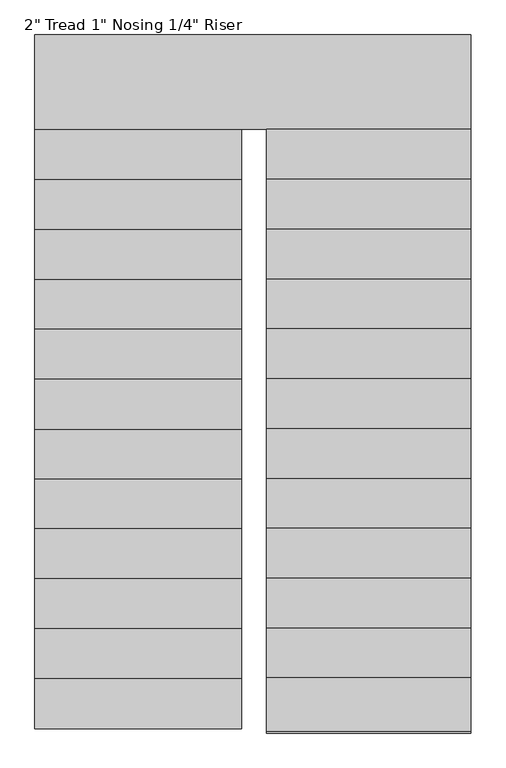
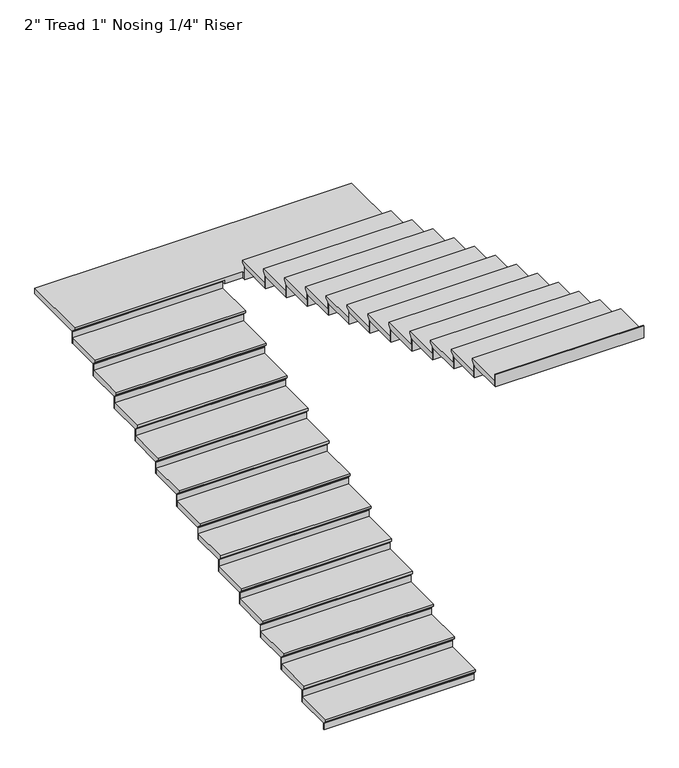
"""IFC4 building model written with IfcOpenShell, lengths in millimetres: stair flight geometry."""

from ifc_helpers import new_model, si_unit, origin, place, context, project, spatial, faceted_brep, source, transform, mapped, element, save


def stair_flight_f068cff5(model_context):
    return source(origin(), model_context, "Body", "Brep", [
        faceted_brep([(-2593.7381751, -9955.5916506, 21422.4576923), (-2593.7381751, -9955.5916506, 21441.5076923), (-3857.687215, -9955.5916506, 21441.5076923), (-3857.687215, -9955.5916506, 21422.4576923), (-2593.7381751, -9930.1916506, 21397.0576923), (-3857.687215, -9930.1916506, 21397.0576923), (-2593.7381751, -9619.0416506, 21441.5076923), (-3857.687215, -9619.0416506, 21441.5076923), (-3857.687215, -9930.1916506, 21390.7076923), (-3857.687215, -9619.0416506, 21390.7076923), (-2593.7381751, -9619.0416506, 21390.7076923), (-2593.7381751, -9930.1916506, 21390.7076923)], [[[0, 1, 2, 3]], [[4, 0, 3, 5]], [[2, 1, 6, 7]], [[8, 9, 10, 11]], [[2, 7, 9, 8, 5, 3]], [[8, 11, 4, 5]], [[6, 1, 0, 4, 11, 10]], [[7, 6, 10, 9]]]),
        faceted_brep([(-2593.7381751, -9930.1916506, 21390.7076923), (-2593.7381751, -9930.1916506, 21336.0), (-2593.7381751, -9923.8416506, 21336.0), (-2593.7381751, -9923.8416506, 21390.7076923), (-3857.687215, -9930.1916506, 21390.7076923), (-3857.687215, -9923.8416506, 21390.7076923), (-3857.687215, -9923.8416506, 21336.0), (-3857.687215, -9930.1916506, 21336.0)], [[[0, 1, 2, 3]], [[4, 5, 6, 7]], [[1, 0, 4, 7]], [[2, 1, 7, 6]], [[3, 2, 6, 5]], [[0, 3, 5, 4]]]),
        faceted_brep([(-2593.7381751, -9619.0416506, 21496.2153846), (-2593.7381751, -9619.0416506, 21390.7076923), (-2593.7381751, -9612.6916506, 21390.7076923), (-2593.7381751, -9612.6916506, 21496.2153846), (-3857.687215, -9619.0416506, 21496.2153846), (-3857.687215, -9612.6916506, 21496.2153846), (-3857.687215, -9612.6916506, 21390.7076923), (-3857.687215, -9619.0416506, 21390.7076923)], [[[0, 1, 2, 3]], [[4, 5, 6, 7]], [[1, 0, 4, 7]], [[2, 1, 7, 6]], [[3, 2, 6, 5]], [[0, 3, 5, 4]]]),
        faceted_brep([(-3857.687215, -9644.4416506, 21547.0153846), (-2593.7381751, -9644.4416506, 21547.0153846), (-2593.7381751, -9314.2416506, 21547.0153846), (-3857.687215, -9314.2416506, 21547.0153846), (-3857.687215, -9619.0416506, 21496.2153846), (-3857.687215, -9314.2416506, 21496.2153846), (-2593.7381751, -9314.2416506, 21496.2153846), (-2593.7381751, -9619.0416506, 21496.2153846), (-3857.687215, -9619.0416506, 21502.5653846), (-3857.687215, -9644.4416506, 21527.9653846), (-2593.7381751, -9619.0416506, 21502.5653846), (-2593.7381751, -9644.4416506, 21527.9653846)], [[[0, 1, 2, 3]], [[4, 5, 6, 7]], [[0, 3, 5, 4, 8, 9]], [[4, 7, 10, 8]], [[2, 1, 11, 10, 7, 6]], [[3, 2, 6, 5]], [[11, 1, 0, 9]], [[10, 11, 9, 8]]]),
        faceted_brep([(-2593.7381751, -9314.2416506, 21601.7230769), (-2593.7381751, -9314.2416506, 21496.2153846), (-2593.7381751, -9307.8916506, 21496.2153846), (-2593.7381751, -9307.8916506, 21601.7230769), (-3857.687215, -9314.2416506, 21601.7230769), (-3857.687215, -9307.8916506, 21601.7230769), (-3857.687215, -9307.8916506, 21496.2153846), (-3857.687215, -9314.2416506, 21496.2153846)], [[[0, 1, 2, 3]], [[4, 5, 6, 7]], [[1, 0, 4, 7]], [[2, 1, 7, 6]], [[3, 2, 6, 5]], [[0, 3, 5, 4]]]),
        faceted_brep([(-3857.687215, -9339.6416506, 21652.5230769), (-2593.7381751, -9339.6416506, 21652.5230769), (-2593.7381751, -9009.4416506, 21652.5230769), (-3857.687215, -9009.4416506, 21652.5230769), (-3857.687215, -9314.2416506, 21601.7230769), (-3857.687215, -9009.4416506, 21601.7230769), (-2593.7381751, -9009.4416506, 21601.7230769), (-2593.7381751, -9314.2416506, 21601.7230769), (-3857.687215, -9314.2416506, 21608.0730769), (-3857.687215, -9339.6416506, 21633.4730769), (-2593.7381751, -9314.2416506, 21608.0730769), (-2593.7381751, -9339.6416506, 21633.4730769)], [[[0, 1, 2, 3]], [[4, 5, 6, 7]], [[0, 3, 5, 4, 8, 9]], [[4, 7, 10, 8]], [[2, 1, 11, 10, 7, 6]], [[3, 2, 6, 5]], [[11, 1, 0, 9]], [[10, 11, 9, 8]]]),
        faceted_brep([(-2593.7381751, -9009.4416506, 21707.2307692), (-2593.7381751, -9009.4416506, 21601.7230769), (-2593.7381751, -9003.0916506, 21601.7230769), (-2593.7381751, -9003.0916506, 21707.2307692), (-3857.687215, -9009.4416506, 21707.2307692), (-3857.687215, -9003.0916506, 21707.2307692), (-3857.687215, -9003.0916506, 21601.7230769), (-3857.687215, -9009.4416506, 21601.7230769)], [[[0, 1, 2, 3]], [[4, 5, 6, 7]], [[1, 0, 4, 7]], [[2, 1, 7, 6]], [[3, 2, 6, 5]], [[0, 3, 5, 4]]]),
        faceted_brep([(-3857.687215, -9034.8416506, 21758.0307692), (-2593.7381751, -9034.8416506, 21758.0307692), (-2593.7381751, -8704.6416506, 21758.0307692), (-3857.687215, -8704.6416506, 21758.0307692), (-3857.687215, -9009.4416506, 21707.2307692), (-3857.687215, -8704.6416506, 21707.2307692), (-2593.7381751, -8704.6416506, 21707.2307692), (-2593.7381751, -9009.4416506, 21707.2307692), (-3857.687215, -9009.4416506, 21713.5807692), (-3857.687215, -9034.8416506, 21738.9807692), (-2593.7381751, -9009.4416506, 21713.5807692), (-2593.7381751, -9034.8416506, 21738.9807692)], [[[0, 1, 2, 3]], [[4, 5, 6, 7]], [[0, 3, 5, 4, 8, 9]], [[4, 7, 10, 8]], [[2, 1, 11, 10, 7, 6]], [[3, 2, 6, 5]], [[11, 1, 0, 9]], [[10, 11, 9, 8]]]),
        faceted_brep([(-2593.7381751, -8704.6416506, 21812.7384615), (-2593.7381751, -8704.6416506, 21707.2307692), (-2593.7381751, -8698.2916506, 21707.2307692), (-2593.7381751, -8698.2916506, 21812.7384615), (-3857.687215, -8704.6416506, 21812.7384615), (-3857.687215, -8698.2916506, 21812.7384615), (-3857.687215, -8698.2916506, 21707.2307692), (-3857.687215, -8704.6416506, 21707.2307692)], [[[0, 1, 2, 3]], [[4, 5, 6, 7]], [[1, 0, 4, 7]], [[2, 1, 7, 6]], [[3, 2, 6, 5]], [[0, 3, 5, 4]]]),
        faceted_brep([(-3857.687215, -8730.0416506, 21863.5384615), (-2593.7381751, -8730.0416506, 21863.5384615), (-2593.7381751, -8399.8416506, 21863.5384615), (-3857.687215, -8399.8416506, 21863.5384615), (-3857.687215, -8704.6416506, 21812.7384615), (-3857.687215, -8399.8416506, 21812.7384615), (-2593.7381751, -8399.8416506, 21812.7384615), (-2593.7381751, -8704.6416506, 21812.7384615), (-3857.687215, -8704.6416506, 21819.0884615), (-3857.687215, -8730.0416506, 21844.4884615), (-2593.7381751, -8704.6416506, 21819.0884615), (-2593.7381751, -8730.0416506, 21844.4884615)], [[[0, 1, 2, 3]], [[4, 5, 6, 7]], [[0, 3, 5, 4, 8, 9]], [[4, 7, 10, 8]], [[2, 1, 11, 10, 7, 6]], [[3, 2, 6, 5]], [[11, 1, 0, 9]], [[10, 11, 9, 8]]]),
        faceted_brep([(-2593.7381751, -8399.8416506, 21918.2461538), (-2593.7381751, -8399.8416506, 21812.7384615), (-2593.7381751, -8393.4916506, 21812.7384615), (-2593.7381751, -8393.4916506, 21918.2461538), (-3857.687215, -8399.8416506, 21918.2461538), (-3857.687215, -8393.4916506, 21918.2461538), (-3857.687215, -8393.4916506, 21812.7384615), (-3857.687215, -8399.8416506, 21812.7384615)], [[[0, 1, 2, 3]], [[4, 5, 6, 7]], [[1, 0, 4, 7]], [[2, 1, 7, 6]], [[3, 2, 6, 5]], [[0, 3, 5, 4]]]),
        faceted_brep([(-3857.687215, -8425.2416506, 21969.0461538), (-2593.7381751, -8425.2416506, 21969.0461538), (-2593.7381751, -8098.2166506, 21969.0461538), (-3857.687215, -8098.2166506, 21969.0461538), (-3857.687215, -8399.8416506, 21918.2461538), (-3857.687215, -8098.2166506, 21918.2461538), (-2593.7381751, -8098.2166506, 21918.2461538), (-2593.7381751, -8399.8416506, 21918.2461538), (-3857.687215, -8399.8416506, 21924.5961538), (-3857.687215, -8425.2416506, 21949.9961538), (-2593.7381751, -8399.8416506, 21924.5961538), (-2593.7381751, -8425.2416506, 21949.9961538)], [[[0, 1, 2, 3]], [[4, 5, 6, 7]], [[0, 3, 5, 4, 8, 9]], [[4, 7, 10, 8]], [[2, 1, 11, 10, 7, 6]], [[3, 2, 6, 5]], [[11, 1, 0, 9]], [[10, 11, 9, 8]]]),
        faceted_brep([(-2593.7381751, -8098.2166506, 22023.7538462), (-2593.7381751, -8098.2166506, 21918.2461538), (-2593.7381751, -8091.8666506, 21918.2461538), (-2593.7381751, -8091.8666506, 22023.7538462), (-3857.687215, -8098.2166506, 22023.7538462), (-3857.687215, -8091.8666506, 22023.7538462), (-3857.687215, -8091.8666506, 21918.2461538), (-3857.687215, -8098.2166506, 21918.2461538)], [[[0, 1, 2, 3]], [[4, 5, 6, 7]], [[1, 0, 4, 7]], [[2, 1, 7, 6]], [[3, 2, 6, 5]], [[0, 3, 5, 4]]]),
        faceted_brep([(-3857.687215, -8123.6166506, 22074.5538462), (-2593.7381751, -8123.6166506, 22074.5538462), (-2593.7381751, -7790.2416506, 22074.5538462), (-3857.687215, -7790.2416506, 22074.5538462), (-3857.687215, -8098.2166506, 22023.7538462), (-3857.687215, -7790.2416506, 22023.7538462), (-2593.7381751, -7790.2416506, 22023.7538462), (-2593.7381751, -8098.2166506, 22023.7538462), (-3857.687215, -8098.2166506, 22030.1038462), (-3857.687215, -8123.6166506, 22055.5038462), (-2593.7381751, -8098.2166506, 22030.1038462), (-2593.7381751, -8123.6166506, 22055.5038462)], [[[0, 1, 2, 3]], [[4, 5, 6, 7]], [[0, 3, 5, 4, 8, 9]], [[4, 7, 10, 8]], [[2, 1, 11, 10, 7, 6]], [[3, 2, 6, 5]], [[11, 1, 0, 9]], [[10, 11, 9, 8]]]),
        faceted_brep([(-2593.7381751, -7790.2416506, 22129.2615385), (-2593.7381751, -7790.2416506, 22023.7538462), (-2593.7381751, -7783.8916506, 22023.7538462), (-2593.7381751, -7783.8916506, 22129.2615385), (-3857.687215, -7790.2416506, 22129.2615385), (-3857.687215, -7783.8916506, 22129.2615385), (-3857.687215, -7783.8916506, 22023.7538462), (-3857.687215, -7790.2416506, 22023.7538462)], [[[0, 1, 2, 3]], [[4, 5, 6, 7]], [[1, 0, 4, 7]], [[2, 1, 7, 6]], [[3, 2, 6, 5]], [[0, 3, 5, 4]]]),
        faceted_brep([(-3857.687215, -7815.6416506, 22180.0615385), (-2593.7381751, -7815.6416506, 22180.0615385), (-2593.7381751, -7485.4416506, 22180.0615385), (-3857.687215, -7485.4416506, 22180.0615385), (-3857.687215, -7790.2416506, 22129.2615385), (-3857.687215, -7485.4416506, 22129.2615385), (-2593.7381751, -7485.4416506, 22129.2615385), (-2593.7381751, -7790.2416506, 22129.2615385), (-3857.687215, -7790.2416506, 22135.6115385), (-3857.687215, -7815.6416506, 22161.0115385), (-2593.7381751, -7790.2416506, 22135.6115385), (-2593.7381751, -7815.6416506, 22161.0115385)], [[[0, 1, 2, 3]], [[4, 5, 6, 7]], [[0, 3, 5, 4, 8, 9]], [[4, 7, 10, 8]], [[2, 1, 11, 10, 7, 6]], [[3, 2, 6, 5]], [[11, 1, 0, 9]], [[10, 11, 9, 8]]]),
        faceted_brep([(-2593.7381751, -7485.4416506, 22234.7692308), (-2593.7381751, -7485.4416506, 22129.2615385), (-2593.7381751, -7479.0916506, 22129.2615385), (-2593.7381751, -7479.0916506, 22234.7692308), (-3857.687215, -7485.4416506, 22234.7692308), (-3857.687215, -7479.0916506, 22234.7692308), (-3857.687215, -7479.0916506, 22129.2615385), (-3857.687215, -7485.4416506, 22129.2615385)], [[[0, 1, 2, 3]], [[4, 5, 6, 7]], [[1, 0, 4, 7]], [[2, 1, 7, 6]], [[3, 2, 6, 5]], [[0, 3, 5, 4]]]),
        faceted_brep([(-3857.687215, -7510.8416506, 22285.5692308), (-2593.7381751, -7510.8416506, 22285.5692308), (-2593.7381751, -7180.6416506, 22285.5692308), (-3857.687215, -7180.6416506, 22285.5692308), (-3857.687215, -7485.4416506, 22234.7692308), (-3857.687215, -7180.6416506, 22234.7692308), (-2593.7381751, -7180.6416506, 22234.7692308), (-2593.7381751, -7485.4416506, 22234.7692308), (-3857.687215, -7485.4416506, 22241.1192308), (-3857.687215, -7510.8416506, 22266.5192308), (-2593.7381751, -7485.4416506, 22241.1192308), (-2593.7381751, -7510.8416506, 22266.5192308)], [[[0, 1, 2, 3]], [[4, 5, 6, 7]], [[0, 3, 5, 4, 8, 9]], [[4, 7, 10, 8]], [[2, 1, 11, 10, 7, 6]], [[3, 2, 6, 5]], [[11, 1, 0, 9]], [[10, 11, 9, 8]]]),
        faceted_brep([(-2593.7381751, -7180.6416506, 22340.2769231), (-2593.7381751, -7180.6416506, 22234.7692308), (-2593.7381751, -7174.2916506, 22234.7692308), (-2593.7381751, -7174.2916506, 22340.2769231), (-3857.687215, -7180.6416506, 22340.2769231), (-3857.687215, -7174.2916506, 22340.2769231), (-3857.687215, -7174.2916506, 22234.7692308), (-3857.687215, -7180.6416506, 22234.7692308)], [[[0, 1, 2, 3]], [[4, 5, 6, 7]], [[1, 0, 4, 7]], [[2, 1, 7, 6]], [[3, 2, 6, 5]], [[0, 3, 5, 4]]]),
        faceted_brep([(-3857.687215, -7206.0416506, 22391.0769231), (-2593.7381751, -7206.0416506, 22391.0769231), (-2593.7381751, -6875.8416506, 22391.0769231), (-3857.687215, -6875.8416506, 22391.0769231), (-3857.687215, -7180.6416506, 22340.2769231), (-3857.687215, -6875.8416506, 22340.2769231), (-2593.7381751, -6875.8416506, 22340.2769231), (-2593.7381751, -7180.6416506, 22340.2769231), (-3857.687215, -7180.6416506, 22346.6269231), (-3857.687215, -7206.0416506, 22372.0269231), (-2593.7381751, -7180.6416506, 22346.6269231), (-2593.7381751, -7206.0416506, 22372.0269231)], [[[0, 1, 2, 3]], [[4, 5, 6, 7]], [[0, 3, 5, 4, 8, 9]], [[4, 7, 10, 8]], [[2, 1, 11, 10, 7, 6]], [[3, 2, 6, 5]], [[11, 1, 0, 9]], [[10, 11, 9, 8]]]),
        faceted_brep([(-2593.7381751, -6875.8416506, 22445.7846154), (-2593.7381751, -6875.8416506, 22340.2769231), (-2593.7381751, -6869.4916506, 22340.2769231), (-2593.7381751, -6869.4916506, 22445.7846154), (-3857.687215, -6875.8416506, 22445.7846154), (-3857.687215, -6869.4916506, 22445.7846154), (-3857.687215, -6869.4916506, 22340.2769231), (-3857.687215, -6875.8416506, 22340.2769231)], [[[0, 1, 2, 3]], [[4, 5, 6, 7]], [[1, 0, 4, 7]], [[2, 1, 7, 6]], [[3, 2, 6, 5]], [[0, 3, 5, 4]]]),
        faceted_brep([(-3857.687215, -6901.2416506, 22496.5846154), (-2593.7381751, -6901.2416506, 22496.5846154), (-2593.7381751, -6571.0416506, 22496.5846154), (-3857.687215, -6571.0416506, 22496.5846154), (-3857.687215, -6875.8416506, 22445.7846154), (-3857.687215, -6571.0416506, 22445.7846154), (-2593.7381751, -6571.0416506, 22445.7846154), (-2593.7381751, -6875.8416506, 22445.7846154), (-3857.687215, -6875.8416506, 22452.1346154), (-3857.687215, -6901.2416506, 22477.5346154), (-2593.7381751, -6875.8416506, 22452.1346154), (-2593.7381751, -6901.2416506, 22477.5346154)], [[[0, 1, 2, 3]], [[4, 5, 6, 7]], [[0, 3, 5, 4, 8, 9]], [[4, 7, 10, 8]], [[2, 1, 11, 10, 7, 6]], [[3, 2, 6, 5]], [[11, 1, 0, 9]], [[10, 11, 9, 8]]]),
        faceted_brep([(-2593.7381751, -6571.0416506, 22551.2923077), (-2593.7381751, -6571.0416506, 22445.7846154), (-2593.7381751, -6564.6916506, 22445.7846154), (-2593.7381751, -6564.6916506, 22551.2923077), (-3857.687215, -6571.0416506, 22551.2923077), (-3857.687215, -6564.6916506, 22551.2923077), (-3857.687215, -6564.6916506, 22445.7846154), (-3857.687215, -6571.0416506, 22445.7846154)], [[[0, 1, 2, 3]], [[4, 5, 6, 7]], [[1, 0, 4, 7]], [[2, 1, 7, 6]], [[3, 2, 6, 5]], [[0, 3, 5, 4]]]),
        faceted_brep([(-3857.687215, -6596.4416506, 22602.0923077), (-2593.7381751, -6596.4416506, 22602.0923077), (-2593.7381751, -6266.2416506, 22602.0923077), (-3857.687215, -6266.2416506, 22602.0923077), (-3857.687215, -6571.0416506, 22551.2923077), (-3857.687215, -6266.2416506, 22551.2923077), (-2593.7381751, -6266.2416506, 22551.2923077), (-2593.7381751, -6571.0416506, 22551.2923077), (-3857.687215, -6571.0416506, 22557.6423077), (-3857.687215, -6596.4416506, 22583.0423077), (-2593.7381751, -6571.0416506, 22557.6423077), (-2593.7381751, -6596.4416506, 22583.0423077)], [[[0, 1, 2, 3]], [[4, 5, 6, 7]], [[0, 3, 5, 4, 8, 9]], [[4, 7, 10, 8]], [[2, 1, 11, 10, 7, 6]], [[3, 2, 6, 5]], [[11, 1, 0, 9]], [[10, 11, 9, 8]]]),
        faceted_brep([(-2593.7381751, -6266.2416506, 22656.8), (-2593.7381751, -6266.2416506, 22551.2923077), (-2593.7381751, -6259.8916506, 22551.2923077), (-2593.7381751, -6259.8916506, 22656.8), (-3857.687215, -6266.2416506, 22656.8), (-3857.687215, -6259.8916506, 22656.8), (-3857.687215, -6259.8916506, 22551.2923077), (-3857.687215, -6266.2416506, 22551.2923077)], [[[0, 1, 2, 3]], [[4, 5, 6, 7]], [[1, 0, 4, 7]], [[2, 1, 7, 6]], [[3, 2, 6, 5]], [[0, 3, 5, 4]]]),
        faceted_brep([(-1190.687215, -6317.0416506, 22707.6), (-1190.687215, -5713.7916506, 22707.6), (-3857.687215, -5713.7916506, 22707.6), (-3857.687215, -6291.6416506, 22707.6), (-2441.3381751, -6291.6416506, 22707.6), (-2441.3381751, -6317.0416506, 22707.6), (-1190.687215, -5713.7916506, 22656.8), (-1190.687215, -6317.0416506, 22656.8), (-2441.3381751, -6317.0416506, 22656.8), (-2441.3381751, -6291.6416506, 22656.8), (-2593.7381751, -6291.6416506, 22656.8), (-2593.7381751, -6266.2416506, 22656.8), (-3857.687215, -6266.2416506, 22656.8), (-3857.687215, -5713.7916506, 22656.8), (-3857.687215, -6266.2416506, 22663.15), (-3857.687215, -6291.6416506, 22688.55), (-2593.7381751, -6266.2416506, 22663.15), (-2593.7381751, -6291.6416506, 22688.55)], [[[0, 1, 2, 3, 4, 5]], [[6, 7, 8, 9, 10, 11, 12, 13]], [[1, 0, 7, 6]], [[2, 1, 6, 13]], [[3, 2, 13, 12, 14, 15]], [[12, 11, 16, 14]], [[11, 10, 17, 16]], [[4, 3, 15, 17, 10, 9]], [[5, 4, 9, 8]], [[0, 5, 8, 7]], [[15, 14, 16, 17]]]),
        faceted_brep([(-2441.3381751, -6317.0416506, 22762.3076923), (-2441.3381751, -6317.0416506, 22656.8), (-2441.3381751, -6323.3916506, 22656.8), (-2441.3381751, -6323.3916506, 22762.3076923), (-1190.687215, -6317.0416506, 22762.3076923), (-1190.687215, -6323.3916506, 22762.3076923), (-1190.687215, -6323.3916506, 22656.8), (-1190.687215, -6317.0416506, 22656.8)], [[[0, 1, 2, 3]], [[4, 5, 6, 7]], [[1, 0, 4, 7]], [[2, 1, 7, 6]], [[3, 2, 6, 5]], [[0, 3, 5, 4]]]),
        faceted_brep([(-1190.687215, -6291.6416506, 22813.1076923), (-2441.3381751, -6291.6416506, 22813.1076923), (-2441.3381751, -6621.8416506, 22813.1076923), (-1190.687215, -6621.8416506, 22813.1076923), (-1190.687215, -6317.0416506, 22762.3076923), (-1190.687215, -6621.8416506, 22762.3076923), (-2441.3381751, -6621.8416506, 22762.3076923), (-2441.3381751, -6317.0416506, 22762.3076923), (-1190.687215, -6317.0416506, 22768.6576923), (-1190.687215, -6291.6416506, 22794.0576923), (-2441.3381751, -6317.0416506, 22768.6576923), (-2441.3381751, -6291.6416506, 22794.0576923)], [[[0, 1, 2, 3]], [[4, 5, 6, 7]], [[0, 3, 5, 4, 8, 9]], [[4, 7, 10, 8]], [[2, 1, 11, 10, 7, 6]], [[3, 2, 6, 5]], [[11, 1, 0, 9]], [[10, 11, 9, 8]]]),
        faceted_brep([(-2441.3381751, -6621.8416506, 22867.8153846), (-2441.3381751, -6621.8416506, 22762.3076923), (-2441.3381751, -6628.1916506, 22762.3076923), (-2441.3381751, -6628.1916506, 22867.8153846), (-1190.687215, -6621.8416506, 22867.8153846), (-1190.687215, -6628.1916506, 22867.8153846), (-1190.687215, -6628.1916506, 22762.3076923), (-1190.687215, -6621.8416506, 22762.3076923)], [[[0, 1, 2, 3]], [[4, 5, 6, 7]], [[1, 0, 4, 7]], [[2, 1, 7, 6]], [[3, 2, 6, 5]], [[0, 3, 5, 4]]]),
        faceted_brep([(-1190.687215, -6596.4416506, 22918.6153846), (-2441.3381751, -6596.4416506, 22918.6153846), (-2441.3381751, -6926.6416506, 22918.6153846), (-1190.687215, -6926.6416506, 22918.6153846), (-1190.687215, -6621.8416506, 22867.8153846), (-1190.687215, -6926.6416506, 22867.8153846), (-2441.3381751, -6926.6416506, 22867.8153846), (-2441.3381751, -6621.8416506, 22867.8153846), (-1190.687215, -6621.8416506, 22874.1653846), (-1190.687215, -6596.4416506, 22899.5653846), (-2441.3381751, -6621.8416506, 22874.1653846), (-2441.3381751, -6596.4416506, 22899.5653846)], [[[0, 1, 2, 3]], [[4, 5, 6, 7]], [[0, 3, 5, 4, 8, 9]], [[4, 7, 10, 8]], [[2, 1, 11, 10, 7, 6]], [[3, 2, 6, 5]], [[11, 1, 0, 9]], [[10, 11, 9, 8]]]),
        faceted_brep([(-2441.3381751, -6926.6416506, 22973.3230769), (-2441.3381751, -6926.6416506, 22867.8153846), (-2441.3381751, -6932.9916506, 22867.8153846), (-2441.3381751, -6932.9916506, 22973.3230769), (-1190.687215, -6926.6416506, 22973.3230769), (-1190.687215, -6932.9916506, 22973.3230769), (-1190.687215, -6932.9916506, 22867.8153846), (-1190.687215, -6926.6416506, 22867.8153846)], [[[0, 1, 2, 3]], [[4, 5, 6, 7]], [[1, 0, 4, 7]], [[2, 1, 7, 6]], [[3, 2, 6, 5]], [[0, 3, 5, 4]]]),
        faceted_brep([(-1190.687215, -6901.2416506, 23024.1230769), (-2441.3381751, -6901.2416506, 23024.1230769), (-2441.3381751, -7231.4416506, 23024.1230769), (-1190.687215, -7231.4416506, 23024.1230769), (-1190.687215, -6926.6416506, 22973.3230769), (-1190.687215, -7231.4416506, 22973.3230769), (-2441.3381751, -7231.4416506, 22973.3230769), (-2441.3381751, -6926.6416506, 22973.3230769), (-1190.687215, -6926.6416506, 22979.6730769), (-1190.687215, -6901.2416506, 23005.0730769), (-2441.3381751, -6926.6416506, 22979.6730769), (-2441.3381751, -6901.2416506, 23005.0730769)], [[[0, 1, 2, 3]], [[4, 5, 6, 7]], [[0, 3, 5, 4, 8, 9]], [[4, 7, 10, 8]], [[2, 1, 11, 10, 7, 6]], [[3, 2, 6, 5]], [[11, 1, 0, 9]], [[10, 11, 9, 8]]]),
        faceted_brep([(-2441.3381751, -7231.4416506, 23078.8307692), (-2441.3381751, -7231.4416506, 22973.3230769), (-2441.3381751, -7237.7916506, 22973.3230769), (-2441.3381751, -7237.7916506, 23078.8307692), (-1190.687215, -7231.4416506, 23078.8307692), (-1190.687215, -7237.7916506, 23078.8307692), (-1190.687215, -7237.7916506, 22973.3230769), (-1190.687215, -7231.4416506, 22973.3230769)], [[[0, 1, 2, 3]], [[4, 5, 6, 7]], [[1, 0, 4, 7]], [[2, 1, 7, 6]], [[3, 2, 6, 5]], [[0, 3, 5, 4]]]),
        faceted_brep([(-1190.687215, -7206.0416506, 23129.6307692), (-2441.3381751, -7206.0416506, 23129.6307692), (-2441.3381751, -7536.2416506, 23129.6307692), (-1190.687215, -7536.2416506, 23129.6307692), (-1190.687215, -7231.4416506, 23078.8307692), (-1190.687215, -7536.2416506, 23078.8307692), (-2441.3381751, -7536.2416506, 23078.8307692), (-2441.3381751, -7231.4416506, 23078.8307692), (-1190.687215, -7231.4416506, 23085.1807692), (-1190.687215, -7206.0416506, 23110.5807692), (-2441.3381751, -7231.4416506, 23085.1807692), (-2441.3381751, -7206.0416506, 23110.5807692)], [[[0, 1, 2, 3]], [[4, 5, 6, 7]], [[0, 3, 5, 4, 8, 9]], [[4, 7, 10, 8]], [[2, 1, 11, 10, 7, 6]], [[3, 2, 6, 5]], [[11, 1, 0, 9]], [[10, 11, 9, 8]]]),
        faceted_brep([(-2441.3381751, -7536.2416506, 23184.3384615), (-2441.3381751, -7536.2416506, 23078.8307692), (-2441.3381751, -7542.5916506, 23078.8307692), (-2441.3381751, -7542.5916506, 23184.3384615), (-1190.687215, -7536.2416506, 23184.3384615), (-1190.687215, -7542.5916506, 23184.3384615), (-1190.687215, -7542.5916506, 23078.8307692), (-1190.687215, -7536.2416506, 23078.8307692)], [[[0, 1, 2, 3]], [[4, 5, 6, 7]], [[1, 0, 4, 7]], [[2, 1, 7, 6]], [[3, 2, 6, 5]], [[0, 3, 5, 4]]]),
        faceted_brep([(-1190.687215, -7510.8416506, 23235.1384615), (-2441.3381751, -7510.8416506, 23235.1384615), (-2441.3381751, -7841.0416506, 23235.1384615), (-1190.687215, -7841.0416506, 23235.1384615), (-1190.687215, -7536.2416506, 23184.3384615), (-1190.687215, -7841.0416506, 23184.3384615), (-2441.3381751, -7841.0416506, 23184.3384615), (-2441.3381751, -7536.2416506, 23184.3384615), (-1190.687215, -7536.2416506, 23190.6884615), (-1190.687215, -7510.8416506, 23216.0884615), (-2441.3381751, -7536.2416506, 23190.6884615), (-2441.3381751, -7510.8416506, 23216.0884615)], [[[0, 1, 2, 3]], [[4, 5, 6, 7]], [[0, 3, 5, 4, 8, 9]], [[4, 7, 10, 8]], [[2, 1, 11, 10, 7, 6]], [[3, 2, 6, 5]], [[11, 1, 0, 9]], [[10, 11, 9, 8]]]),
        faceted_brep([(-2441.3381751, -7841.0416506, 23289.8461538), (-2441.3381751, -7841.0416506, 23184.3384615), (-2441.3381751, -7847.3916506, 23184.3384615), (-2441.3381751, -7847.3916506, 23289.8461538), (-1190.687215, -7841.0416506, 23289.8461538), (-1190.687215, -7847.3916506, 23289.8461538), (-1190.687215, -7847.3916506, 23184.3384615), (-1190.687215, -7841.0416506, 23184.3384615)], [[[0, 1, 2, 3]], [[4, 5, 6, 7]], [[1, 0, 4, 7]], [[2, 1, 7, 6]], [[3, 2, 6, 5]], [[0, 3, 5, 4]]]),
        faceted_brep([(-1190.687215, -7815.6416506, 23340.6461538), (-2441.3381751, -7815.6416506, 23340.6461538), (-2441.3381751, -8145.8416506, 23340.6461538), (-1190.687215, -8145.8416506, 23340.6461538), (-1190.687215, -7841.0416506, 23289.8461538), (-1190.687215, -8145.8416506, 23289.8461538), (-2441.3381751, -8145.8416506, 23289.8461538), (-2441.3381751, -7841.0416506, 23289.8461538), (-1190.687215, -7841.0416506, 23296.1961538), (-1190.687215, -7815.6416506, 23321.5961538), (-2441.3381751, -7841.0416506, 23296.1961538), (-2441.3381751, -7815.6416506, 23321.5961538)], [[[0, 1, 2, 3]], [[4, 5, 6, 7]], [[0, 3, 5, 4, 8, 9]], [[4, 7, 10, 8]], [[2, 1, 11, 10, 7, 6]], [[3, 2, 6, 5]], [[11, 1, 0, 9]], [[10, 11, 9, 8]]]),
        faceted_brep([(-2441.3381751, -8145.8416506, 23395.3538462), (-2441.3381751, -8145.8416506, 23289.8461538), (-2441.3381751, -8152.1916506, 23289.8461538), (-2441.3381751, -8152.1916506, 23395.3538462), (-1190.687215, -8145.8416506, 23395.3538462), (-1190.687215, -8152.1916506, 23395.3538462), (-1190.687215, -8152.1916506, 23289.8461538), (-1190.687215, -8145.8416506, 23289.8461538)], [[[0, 1, 2, 3]], [[4, 5, 6, 7]], [[1, 0, 4, 7]], [[2, 1, 7, 6]], [[3, 2, 6, 5]], [[0, 3, 5, 4]]]),
        faceted_brep([(-1190.687215, -8120.4416506, 23446.1538462), (-2441.3381751, -8120.4416506, 23446.1538462), (-2441.3381751, -8450.6416506, 23446.1538462), (-1190.687215, -8450.6416506, 23446.1538462), (-1190.687215, -8145.8416506, 23395.3538462), (-1190.687215, -8450.6416506, 23395.3538462), (-2441.3381751, -8450.6416506, 23395.3538462), (-2441.3381751, -8145.8416506, 23395.3538462), (-1190.687215, -8145.8416506, 23401.7038462), (-1190.687215, -8120.4416506, 23427.1038462), (-2441.3381751, -8145.8416506, 23401.7038462), (-2441.3381751, -8120.4416506, 23427.1038462)], [[[0, 1, 2, 3]], [[4, 5, 6, 7]], [[0, 3, 5, 4, 8, 9]], [[4, 7, 10, 8]], [[2, 1, 11, 10, 7, 6]], [[3, 2, 6, 5]], [[11, 1, 0, 9]], [[10, 11, 9, 8]]]),
        faceted_brep([(-2441.3381751, -8450.6416506, 23500.8615385), (-2441.3381751, -8450.6416506, 23395.3538462), (-2441.3381751, -8456.9916506, 23395.3538462), (-2441.3381751, -8456.9916506, 23500.8615385), (-1190.687215, -8450.6416506, 23500.8615385), (-1190.687215, -8456.9916506, 23500.8615385), (-1190.687215, -8456.9916506, 23395.3538462), (-1190.687215, -8450.6416506, 23395.3538462)], [[[0, 1, 2, 3]], [[4, 5, 6, 7]], [[1, 0, 4, 7]], [[2, 1, 7, 6]], [[3, 2, 6, 5]], [[0, 3, 5, 4]]]),
        faceted_brep([(-1190.687215, -8425.2416506, 23551.6615385), (-2441.3381751, -8425.2416506, 23551.6615385), (-2441.3381751, -8755.4416506, 23551.6615385), (-1190.687215, -8755.4416506, 23551.6615385), (-1190.687215, -8450.6416506, 23500.8615385), (-1190.687215, -8755.4416506, 23500.8615385), (-2441.3381751, -8755.4416506, 23500.8615385), (-2441.3381751, -8450.6416506, 23500.8615385), (-1190.687215, -8450.6416506, 23507.2115385), (-1190.687215, -8425.2416506, 23532.6115385), (-2441.3381751, -8450.6416506, 23507.2115385), (-2441.3381751, -8425.2416506, 23532.6115385)], [[[0, 1, 2, 3]], [[4, 5, 6, 7]], [[0, 3, 5, 4, 8, 9]], [[4, 7, 10, 8]], [[2, 1, 11, 10, 7, 6]], [[3, 2, 6, 5]], [[11, 1, 0, 9]], [[10, 11, 9, 8]]]),
        faceted_brep([(-2441.3381751, -8755.4416506, 23606.3692308), (-2441.3381751, -8755.4416506, 23500.8615385), (-2441.3381751, -8761.7916506, 23500.8615385), (-2441.3381751, -8761.7916506, 23606.3692308), (-1190.687215, -8755.4416506, 23606.3692308), (-1190.687215, -8761.7916506, 23606.3692308), (-1190.687215, -8761.7916506, 23500.8615385), (-1190.687215, -8755.4416506, 23500.8615385)], [[[0, 1, 2, 3]], [[4, 5, 6, 7]], [[1, 0, 4, 7]], [[2, 1, 7, 6]], [[3, 2, 6, 5]], [[0, 3, 5, 4]]]),
        faceted_brep([(-1190.687215, -8730.0416506, 23657.1692308), (-2441.3381751, -8730.0416506, 23657.1692308), (-2441.3381751, -9060.2416506, 23657.1692308), (-1190.687215, -9060.2416506, 23657.1692308), (-1190.687215, -8755.4416506, 23606.3692308), (-1190.687215, -9060.2416506, 23606.3692308), (-2441.3381751, -9060.2416506, 23606.3692308), (-2441.3381751, -8755.4416506, 23606.3692308), (-1190.687215, -8755.4416506, 23612.7192308), (-1190.687215, -8730.0416506, 23638.1192308), (-2441.3381751, -8755.4416506, 23612.7192308), (-2441.3381751, -8730.0416506, 23638.1192308)], [[[0, 1, 2, 3]], [[4, 5, 6, 7]], [[0, 3, 5, 4, 8, 9]], [[4, 7, 10, 8]], [[2, 1, 11, 10, 7, 6]], [[3, 2, 6, 5]], [[11, 1, 0, 9]], [[10, 11, 9, 8]]]),
        faceted_brep([(-2441.3381751, -9060.2416506, 23711.8769231), (-2441.3381751, -9060.2416506, 23606.3692308), (-2441.3381751, -9066.5916506, 23606.3692308), (-2441.3381751, -9066.5916506, 23711.8769231), (-1190.687215, -9060.2416506, 23711.8769231), (-1190.687215, -9066.5916506, 23711.8769231), (-1190.687215, -9066.5916506, 23606.3692308), (-1190.687215, -9060.2416506, 23606.3692308)], [[[0, 1, 2, 3]], [[4, 5, 6, 7]], [[1, 0, 4, 7]], [[2, 1, 7, 6]], [[3, 2, 6, 5]], [[0, 3, 5, 4]]]),
        faceted_brep([(-1190.687215, -9034.8416506, 23762.6769231), (-2441.3381751, -9034.8416506, 23762.6769231), (-2441.3381751, -9365.0416506, 23762.6769231), (-1190.687215, -9365.0416506, 23762.6769231), (-1190.687215, -9060.2416506, 23711.8769231), (-1190.687215, -9365.0416506, 23711.8769231), (-2441.3381751, -9365.0416506, 23711.8769231), (-2441.3381751, -9060.2416506, 23711.8769231), (-1190.687215, -9060.2416506, 23718.2269231), (-1190.687215, -9034.8416506, 23743.6269231), (-2441.3381751, -9060.2416506, 23718.2269231), (-2441.3381751, -9034.8416506, 23743.6269231)], [[[0, 1, 2, 3]], [[4, 5, 6, 7]], [[0, 3, 5, 4, 8, 9]], [[4, 7, 10, 8]], [[2, 1, 11, 10, 7, 6]], [[3, 2, 6, 5]], [[11, 1, 0, 9]], [[10, 11, 9, 8]]]),
        faceted_brep([(-2441.3381751, -9365.0416506, 23817.3846154), (-2441.3381751, -9365.0416506, 23711.8769231), (-2441.3381751, -9371.3916506, 23711.8769231), (-2441.3381751, -9371.3916506, 23817.3846154), (-1190.687215, -9365.0416506, 23817.3846154), (-1190.687215, -9371.3916506, 23817.3846154), (-1190.687215, -9371.3916506, 23711.8769231), (-1190.687215, -9365.0416506, 23711.8769231)], [[[0, 1, 2, 3]], [[4, 5, 6, 7]], [[1, 0, 4, 7]], [[2, 1, 7, 6]], [[3, 2, 6, 5]], [[0, 3, 5, 4]]]),
        faceted_brep([(-1190.687215, -9339.6416506, 23868.1846154), (-2441.3381751, -9339.6416506, 23868.1846154), (-2441.3381751, -9669.8416506, 23868.1846154), (-1190.687215, -9669.8416506, 23868.1846154), (-1190.687215, -9365.0416506, 23817.3846154), (-1190.687215, -9669.8416506, 23817.3846154), (-2441.3381751, -9669.8416506, 23817.3846154), (-2441.3381751, -9365.0416506, 23817.3846154), (-1190.687215, -9365.0416506, 23823.7346154), (-1190.687215, -9339.6416506, 23849.1346154), (-2441.3381751, -9365.0416506, 23823.7346154), (-2441.3381751, -9339.6416506, 23849.1346154)], [[[0, 1, 2, 3]], [[4, 5, 6, 7]], [[0, 3, 5, 4, 8, 9]], [[4, 7, 10, 8]], [[2, 1, 11, 10, 7, 6]], [[3, 2, 6, 5]], [[11, 1, 0, 9]], [[10, 11, 9, 8]]]),
        faceted_brep([(-2441.3381751, -9669.8416506, 23922.8923077), (-2441.3381751, -9669.8416506, 23817.3846154), (-2441.3381751, -9676.1916506, 23817.3846154), (-2441.3381751, -9676.1916506, 23922.8923077), (-1190.687215, -9669.8416506, 23922.8923077), (-1190.687215, -9676.1916506, 23922.8923077), (-1190.687215, -9676.1916506, 23817.3846154), (-1190.687215, -9669.8416506, 23817.3846154)], [[[0, 1, 2, 3]], [[4, 5, 6, 7]], [[1, 0, 4, 7]], [[2, 1, 7, 6]], [[3, 2, 6, 5]], [[0, 3, 5, 4]]]),
        faceted_brep([(-2441.3381751, -9974.6416506, 24028.4), (-2441.3381751, -9974.6416506, 23922.8923077), (-2441.3381751, -9980.9916506, 23922.8923077), (-2441.3381751, -9980.9916506, 24028.4), (-1190.687215, -9974.6416506, 24028.4), (-1190.687215, -9980.9916506, 24028.4), (-1190.687215, -9980.9916506, 23922.8923077), (-1190.687215, -9974.6416506, 23922.8923077)], [[[0, 1, 2, 3]], [[4, 5, 6, 7]], [[1, 0, 4, 7]], [[2, 1, 7, 6]], [[3, 2, 6, 5]], [[0, 3, 5, 4]]]),
        faceted_brep([(-1190.687215, -9644.4416506, 23973.6923077), (-2441.3381751, -9644.4416506, 23973.6923077), (-2441.3381751, -9974.6416506, 23973.6923077), (-1190.687215, -9974.6416506, 23973.6923077), (-1190.687215, -9669.8416506, 23922.8923077), (-1190.687215, -9974.6416506, 23922.8923077), (-2441.3381751, -9974.6416506, 23922.8923077), (-2441.3381751, -9669.8416506, 23922.8923077), (-1190.687215, -9669.8416506, 23929.2423077), (-1190.687215, -9644.4416506, 23954.6423077), (-2441.3381751, -9669.8416506, 23929.2423077), (-2441.3381751, -9644.4416506, 23954.6423077)], [[[0, 1, 2, 3]], [[4, 5, 6, 7]], [[0, 3, 5, 4, 8, 9]], [[4, 7, 10, 8]], [[2, 1, 11, 10, 7, 6]], [[3, 2, 6, 5]], [[11, 1, 0, 9]], [[10, 11, 9, 8]]]),
    ])


if __name__ == "__main__":
    model = new_model("IFC4")
    model_context = context("Model", 3, world=origin())
    ifc_project = project(units=[si_unit("LENGTHUNIT", "METRE", prefix="MILLI")], contexts=[model_context])
    site = spatial("IfcSite", under=ifc_project)
    building = spatial("IfcBuilding", under=site)
    placement = place(None, origin())
    stair_flight_shape = stair_flight_f068cff5(model_context)
    element("IfcStairFlight", 1, ObjectType="2\" Tread 1\" Nosing 1/4\" Riser", at=placement, inside=building, context=model_context, shape_type="MappedRepresentation", body=[
        mapped(stair_flight_shape, transform((0.0, 0.0, 0.0), x_axis=(1.0, 0.0, 0.0), y_axis=(0.0, 1.0, 0.0), z_axis=(0.0, 0.0, 1.0))),
    ])
    save(model, "model.ifc")
